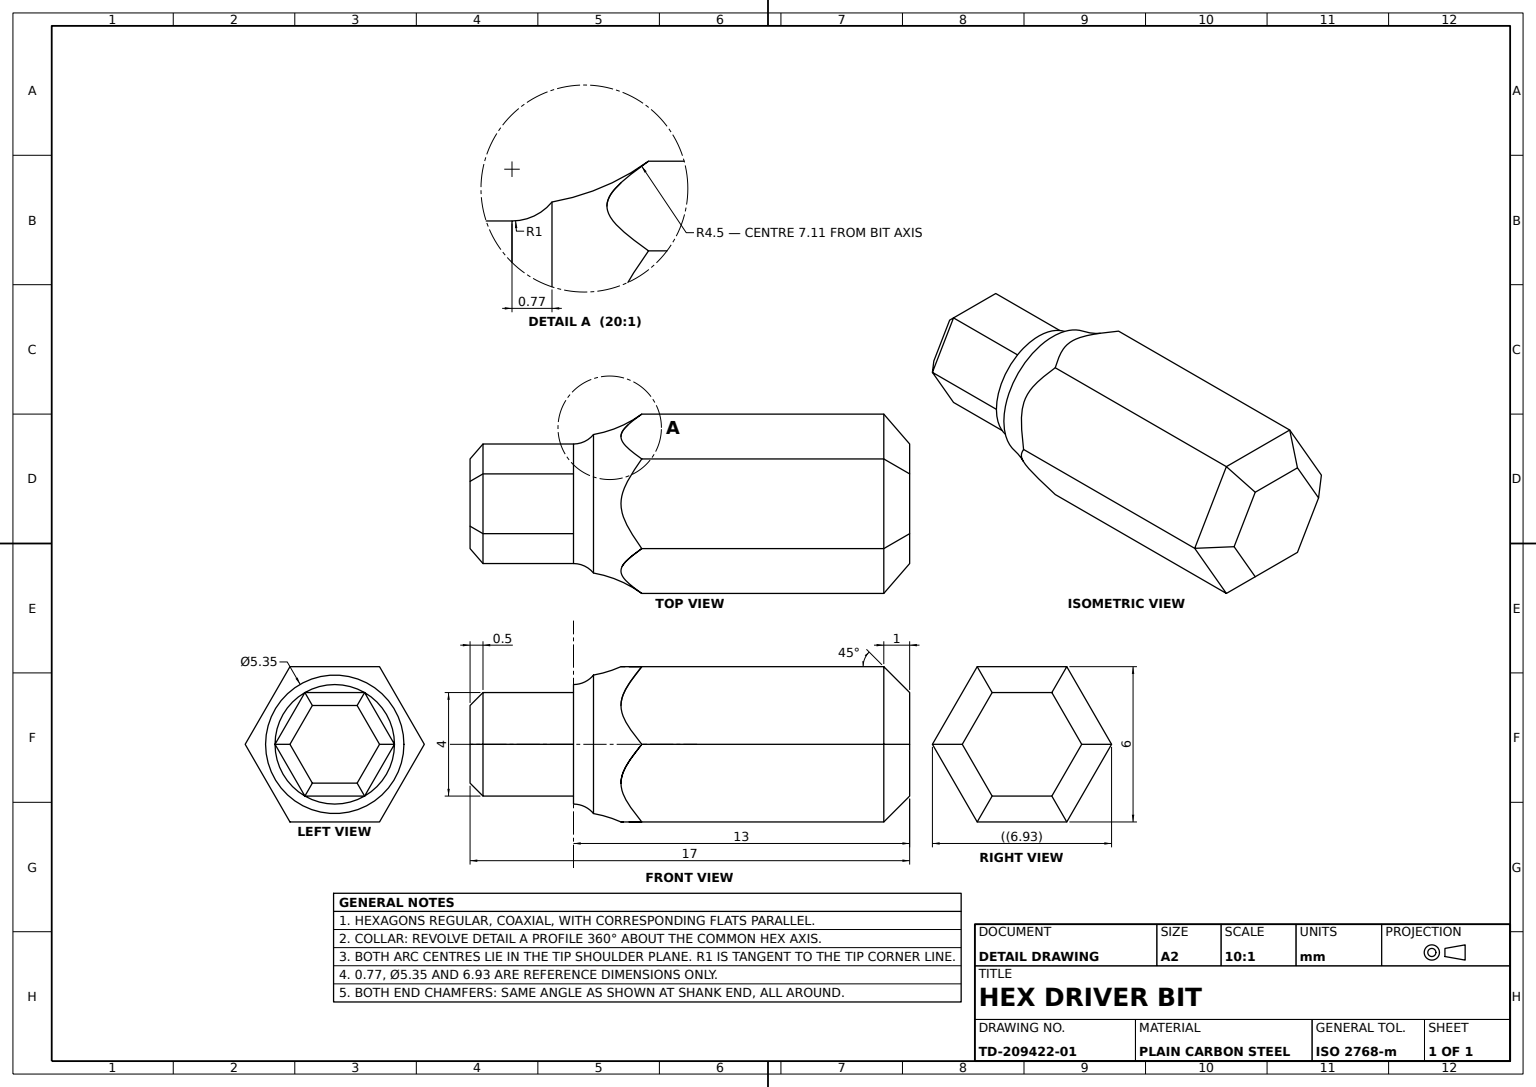
from build123d import *

# Parameters (mm, degrees)
HEX_SHANK_6AF_X13_DEPTH   = 13
HEX_TIP_4AF_X4_DEPTH      = 4
HEX_TIP_4AF_X4_DEPTH_BACK = 4
TIP_CHAMFER_0_5_SIZE      = 0.5
SHANK_CHAMFER_1_SIZE      = 1


with BuildPart() as part:
    # Hex Shank Profile 6AF → Hex Shank 6AF x13 (new body)
    with BuildSketch(Plane.XY):
        Polygon((3.464101615, 0), (1.732050808, 3), (-1.732050808, 3), (-3.464101615, 0), (-1.732050808, -3), (1.732050808, -3), align=None)
    extrude(amount=HEX_SHANK_6AF_X13_DEPTH)

    # Hex Tip Profile 4AF → Hex Tip 4AF x4 (add, two sides: drawn at the far end of the back side and taken through both)
    with BuildSketch(Plane.XY.offset(13).offset(-HEX_TIP_4AF_X4_DEPTH_BACK)):
        Polygon((2.309401077, 0), (1.154700538, 2), (-1.154700538, 2), (-2.309401077, 0), (-1.154700538, -2), (1.154700538, -2), align=None)
    extrude(amount=HEX_TIP_4AF_X4_DEPTH + HEX_TIP_4AF_X4_DEPTH_BACK)

    # Neck Groove Profile → Neck Groove (revolve, cut)
    with BuildSketch(Plane(origin=(0, 0, 0), x_dir=(1, 0, 0), z_dir=(0, 1, 0)), mode=Mode.PRIVATE) as neck_groove_sk:
        with BuildLine():
            Line((3.464101615, -10.360098242), (3.464101615, -13))
            Line((3.464101615, -13), (2.309401077, -13))
            ThreePointArc((2.309401077, -13), (2.40550356, -12.572250915), (2.675339636, -12.226717329))
            ThreePointArc((2.675339636, -12.226717329), (2.963282684, -11.248431174), (3.464101615, -10.360098242))
        make_face()
    revolve(neck_groove_sk.sketch.rotate(Axis((0, 0, 0), (0, 0, 1)), 180), axis=Axis((0, 0, 0), (0, 0, 1)), mode=Mode.SUBTRACT)

    # Tip Chamfer 0.5
    tip_chamfer_0_5_edges = [part.edges().sort_by_distance(p)[0] for p in [
        (1.732050808, -1, 17),
        (1.732050808, 1, 17),
        (0, 2, 17),
        (-1.732050808, 1, 17),
        (-1.732050808, -1, 17),
        (0, -2, 17),
    ]]
    chamfer(tip_chamfer_0_5_edges, length=TIP_CHAMFER_0_5_SIZE)

    # Shank Chamfer 1
    shank_chamfer_1_edges = [part.edges().sort_by_distance(p)[0] for p in [
        (0, -3, 0),
        (-2.598076211, -1.5, 0),
        (-2.598076211, 1.5, 0),
        (0, 3, 0),
        (2.598076211, 1.5, 0),
        (2.598076211, -1.5, 0),
    ]]
    chamfer(shank_chamfer_1_edges, length=SHANK_CHAMFER_1_SIZE)


solid = part.part
